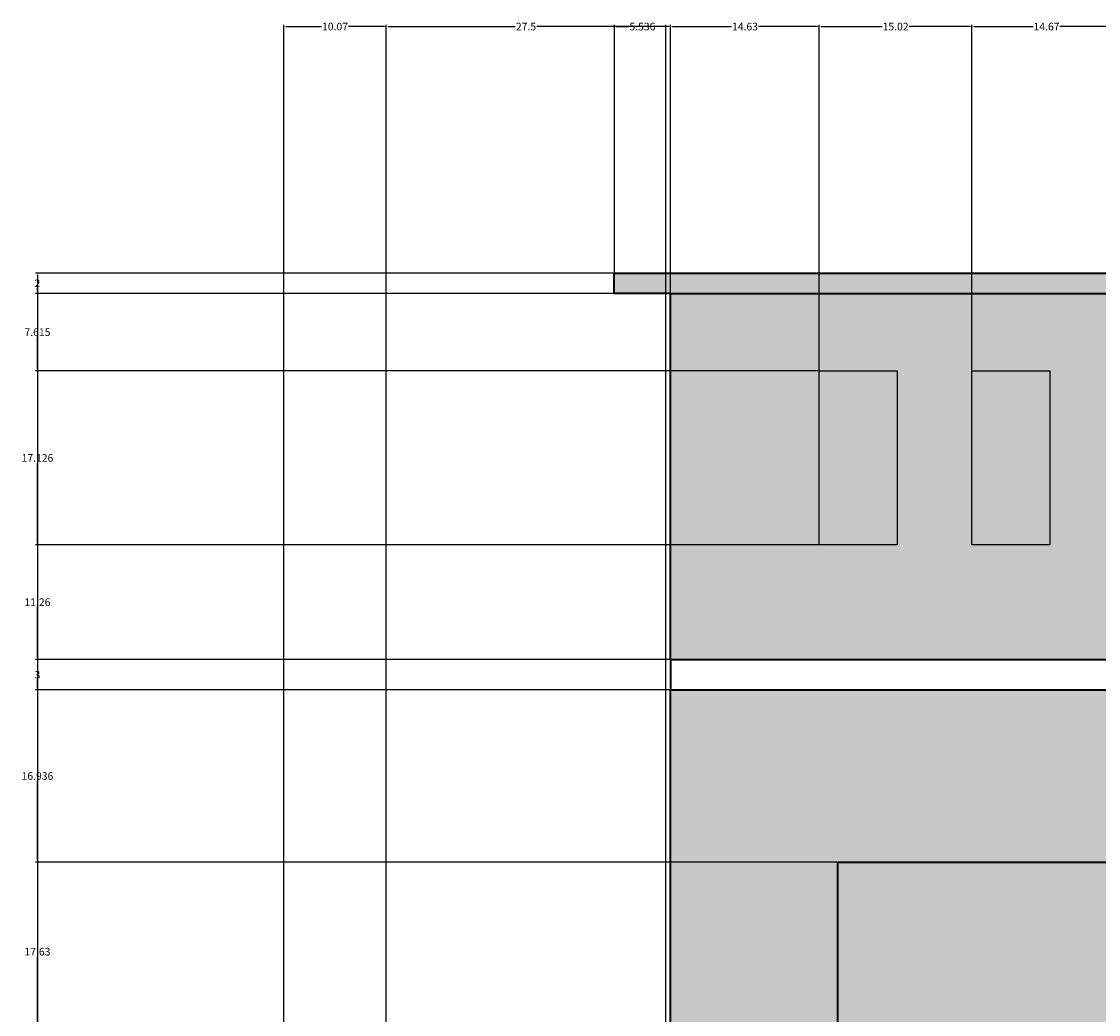
# Model space of a CAD drawing. Units: inches. Extents: x 62 to 566, y 66 to 528.
# Tile 9 of 20: x 62 to 168, y 430 to 528. Entities that reach past the tile are written whole.
import ezdxf

# ---------------------------------------------------------------- set-up
doc = ezdxf.new("R2010")
doc.units = ezdxf.units.IN
doc.header["$MEASUREMENT"] = 0
for name, color, linetype, lineweight in [('A-ANNO-DIMS', 2, 'Continuous', 18), ('A-ELEV', 7, 'Continuous', 35), ('A-GLAZ', 3, 'Continuous', 25), ('A-WALL-PATT', 8, 'Continuous', 13)]:
    doc.layers.add(name, color=color, linetype=linetype, lineweight=lineweight)
doc.styles.get("Standard").update_dxf_attribs({"font": 'arial.ttf'})
doc.dimstyles.get("Standard").update_dxf_attribs({"dimtxt": 0.75, "dimasz": 0.18, "dimexe": 0.18, "dimexo": 0.0625, "dimgap": 0.09, "dimtad": 0, "dimtih": 1, "dimtoh": 1, "dimdec": 4, "dimzin": 0, "dimdsep": 46, "dimlunit": 4, "dimtxsty": 'Standard', "dimcen": 0.09, "dimadec": 0, "dimazin": 0, "dimtfac": 1, "dimtdec": 4, "dimtofl": 0, "dimtmove": 0, "dimatfit": 3, "dimfxl": 1, "dimtolj": 1, "dimtzin": 0, "dimarcsym": 0})

# ---------------------------------------------------------------- blocks, each defined once
blk = doc.blocks.new('VENT-OPENING')
blk.add_lwpolyline([(0, 17.13), (7.66, 17.13), (7.66, 0), (0, 0)], close=True)
blk = doc.blocks.new('*D14')
at = {"layer": 'A-ANNO-DIMS', "color": 0, "lineweight": -2, "transparency": 16777216}
for p, q in [((87.9, 174.13), (87.9, 527.47)), ((88.08, 527.29), (91.61, 527.29)), ((97.79, 527.29), (94.25, 527.29)), ((97.97, 174.13), (97.97, 527.47))]:
    blk.add_line(p, q, dxfattribs=at)
at = {"layer": 'A-ANNO-DIMS', "color": 0, "transparency": 16777216}
for points in [[(88.08, 527.32), (88.08, 527.26), (87.9, 527.29)], [(97.79, 527.32), (97.79, 527.26), (97.97, 527.29)]]:
    blk.add_solid(points, dxfattribs=at)
at = {"layer": 'Defpoints', "color": 0, "transparency": 16777216}
for p in [(97.97, 527.29), (87.9, 174.07), (97.97, 174.07)]:
    blk.add_point(p, dxfattribs=at)
at = {"layer": 'A-ANNO-DIMS', "color": 0, "transparency": 16777216, "insert": (92.93, 527.29), "char_height": 0.75, "attachment_point": 5}
blk.add_mtext('\\A1;10.07', dxfattribs=at)
blk = doc.blocks.new('*D15')
at = {"layer": 'A-ANNO-DIMS', "color": 0, "lineweight": -2, "transparency": 16777216}
for p, q in [((97.97, 174.13), (97.97, 527.47)), ((98.15, 527.29), (110.64, 527.29)), ((125.28, 527.29), (112.79, 527.29)), ((125.46, 174.13), (125.46, 527.47))]:
    blk.add_line(p, q, dxfattribs=at)
at = {"layer": 'A-ANNO-DIMS', "color": 0, "transparency": 16777216}
for points in [[(98.15, 527.32), (98.15, 527.26), (97.97, 527.29)], [(125.28, 527.32), (125.28, 527.26), (125.46, 527.29)]]:
    blk.add_solid(points, dxfattribs=at)
at = {"layer": 'Defpoints', "color": 0, "transparency": 16777216}
for p in [(125.46, 527.29), (97.97, 174.07), (125.46, 174.07)]:
    blk.add_point(p, dxfattribs=at)
at = {"layer": 'A-ANNO-DIMS', "color": 0, "transparency": 16777216, "insert": (111.72, 527.29), "char_height": 0.75, "attachment_point": 5}
blk.add_mtext('\\A1;27.5', dxfattribs=at)
blk = doc.blocks.new('*D18')
at = {"layer": 'A-ANNO-DIMS', "color": 0, "lineweight": -2, "transparency": 16777216}
for p, q in [((120.34, 503.04), (63.47, 503.04)), ((63.65, 502.86), (63.65, 339.03)), ((63.65, 174.25), (63.65, 338.08)), ((87.83, 174.07), (63.47, 174.07))]:
    blk.add_line(p, q, dxfattribs=at)
at = {"layer": 'A-ANNO-DIMS', "color": 0, "transparency": 16777216}
for points in [[(63.62, 502.86), (63.68, 502.86), (63.65, 503.04)], [(63.62, 174.25), (63.68, 174.25), (63.65, 174.07)]]:
    blk.add_solid(points, dxfattribs=at)
at = {"layer": 'Defpoints', "color": 0, "transparency": 16777216}
for p in [(63.65, 503.04), (120.41, 503.04), (87.9, 174.07)]:
    blk.add_point(p, dxfattribs=at)
at = {"layer": 'A-ANNO-DIMS', "color": 0, "transparency": 16777216, "insert": (63.65, 338.55), "char_height": 0.75, "attachment_point": 5}
blk.add_mtext('\\A1;329', dxfattribs=at)
blk = doc.blocks.new('*D25')
at = {"layer": 'A-ANNO-DIMS', "color": 0, "lineweight": -2, "transparency": 16777216}
for p, q in [((120.41, 503.1), (120.41, 527.47)), ((120.59, 527.29), (121.82, 527.29)), ((125.76, 527.29), (124.53, 527.29)), ((125.94, 501.1), (125.94, 527.47))]:
    blk.add_line(p, q, dxfattribs=at)
at = {"layer": 'A-ANNO-DIMS', "color": 0, "transparency": 16777216}
for points in [[(120.59, 527.32), (120.59, 527.26), (120.41, 527.29)], [(125.76, 527.32), (125.76, 527.26), (125.94, 527.29)]]:
    blk.add_solid(points, dxfattribs=at)
at = {"layer": 'Defpoints', "color": 0, "transparency": 16777216}
for p in [(125.94, 527.29), (120.41, 503.04), (125.94, 501.04)]:
    blk.add_point(p, dxfattribs=at)
at = {"layer": 'A-ANNO-DIMS', "color": 0, "transparency": 16777216, "insert": (123.17, 527.29), "char_height": 0.75, "attachment_point": 5}
blk.add_mtext('\\A1;5.536', dxfattribs=at)
blk = doc.blocks.new('*D26')
at = {"layer": 'A-ANNO-DIMS', "color": 0, "lineweight": -2, "transparency": 16777216}
for p, q in [((125.94, 501.1), (125.94, 527.47)), ((126.12, 527.29), (131.94, 527.29)), ((140.39, 527.29), (134.58, 527.29)), ((140.57, 493.49), (140.57, 527.47))]:
    blk.add_line(p, q, dxfattribs=at)
at = {"layer": 'A-ANNO-DIMS', "color": 0, "transparency": 16777216}
for points in [[(126.12, 527.32), (126.12, 527.26), (125.94, 527.29)], [(140.39, 527.32), (140.39, 527.26), (140.57, 527.29)]]:
    blk.add_solid(points, dxfattribs=at)
at = {"layer": 'Defpoints', "color": 0, "transparency": 16777216}
for p in [(140.57, 527.29), (125.94, 501.04), (140.57, 493.43)]:
    blk.add_point(p, dxfattribs=at)
at = {"layer": 'A-ANNO-DIMS', "color": 0, "transparency": 16777216, "insert": (133.26, 527.29), "char_height": 0.75, "attachment_point": 5}
blk.add_mtext('\\A1;14.63', dxfattribs=at)
blk = doc.blocks.new('*D27')
at = {"layer": 'A-ANNO-DIMS', "color": 0, "lineweight": -2, "transparency": 16777216}
for p, q in [((140.57, 493.49), (140.57, 527.47)), ((140.75, 527.29), (146.76, 527.29)), ((155.41, 527.29), (149.4, 527.29)), ((155.59, 493.49), (155.59, 527.47))]:
    blk.add_line(p, q, dxfattribs=at)
at = {"layer": 'A-ANNO-DIMS', "color": 0, "transparency": 16777216}
for points in [[(140.75, 527.32), (140.75, 527.26), (140.57, 527.29)], [(155.41, 527.32), (155.41, 527.26), (155.59, 527.29)]]:
    blk.add_solid(points, dxfattribs=at)
at = {"layer": 'Defpoints', "color": 0, "transparency": 16777216}
for p in [(155.59, 527.29), (140.57, 493.43), (155.59, 493.43)]:
    blk.add_point(p, dxfattribs=at)
at = {"layer": 'A-ANNO-DIMS', "color": 0, "transparency": 16777216, "insert": (148.08, 527.29), "char_height": 0.75, "attachment_point": 5}
blk.add_mtext('\\A1;15.02', dxfattribs=at)
blk = doc.blocks.new('*D28')
at = {"layer": 'A-ANNO-DIMS', "color": 0, "lineweight": -2, "transparency": 16777216}
for p, q in [((155.59, 493.49), (155.59, 527.47)), ((155.77, 527.29), (161.61, 527.29)), ((170.08, 527.29), (164.25, 527.29)), ((170.26, 493.84), (170.26, 527.47))]:
    blk.add_line(p, q, dxfattribs=at)
at = {"layer": 'A-ANNO-DIMS', "color": 0, "transparency": 16777216}
for points in [[(155.77, 527.32), (155.77, 527.26), (155.59, 527.29)], [(170.08, 527.32), (170.08, 527.26), (170.26, 527.29)]]:
    blk.add_solid(points, dxfattribs=at)
at = {"layer": 'Defpoints', "color": 0, "transparency": 16777216}
for p in [(170.26, 527.29), (170.26, 493.78), (155.59, 493.43)]:
    blk.add_point(p, dxfattribs=at)
at = {"layer": 'A-ANNO-DIMS', "color": 0, "transparency": 16777216, "insert": (162.93, 527.29), "char_height": 0.75, "attachment_point": 5}
blk.add_mtext('\\A1;14.67', dxfattribs=at)
blk = doc.blocks.new('*D35')
at = {"layer": 'A-ANNO-DIMS', "color": 0, "lineweight": -2, "transparency": 16777216}
for p, q in [((125.94, 461.98), (125.94, 65.94)), ((142.39, 445.04), (142.39, 65.94)), ((126.12, 66.12), (132.55, 66.12)), ((142.21, 66.12), (135.77, 66.12))]:
    blk.add_line(p, q, dxfattribs=at)
at = {"layer": 'A-ANNO-DIMS', "color": 0, "transparency": 16777216}
for points in [[(126.12, 66.15), (126.12, 66.09), (125.94, 66.12)], [(142.21, 66.15), (142.21, 66.09), (142.39, 66.12)]]:
    blk.add_solid(points, dxfattribs=at)
at = {"layer": 'Defpoints', "color": 0, "transparency": 16777216}
for p in [(125.94, 462.04), (142.39, 445.11), (142.39, 66.12)]:
    blk.add_point(p, dxfattribs=at)
at = {"layer": 'A-ANNO-DIMS', "color": 0, "transparency": 16777216, "insert": (134.16, 66.12), "char_height": 0.75, "attachment_point": 5}
blk.add_mtext('\\A1;16.443', dxfattribs=at)
blk = doc.blocks.new('*D36')
at = {"layer": 'A-ANNO-DIMS', "color": 0, "lineweight": -2, "transparency": 16777216}
for p, q in [((142.39, 445.04), (142.39, 65.94)), ((163.65, 427.41), (163.65, 65.94)), ((142.57, 66.12), (151.66, 66.12)), ((163.47, 66.12), (154.38, 66.12))]:
    blk.add_line(p, q, dxfattribs=at)
at = {"layer": 'A-ANNO-DIMS', "color": 0, "transparency": 16777216}
for points in [[(142.57, 66.15), (142.57, 66.09), (142.39, 66.12)], [(163.47, 66.15), (163.47, 66.09), (163.65, 66.12)]]:
    blk.add_solid(points, dxfattribs=at)
at = {"layer": 'Defpoints', "color": 0, "transparency": 16777216}
for p in [(142.39, 445.11), (163.65, 427.48), (163.65, 66.12)]:
    blk.add_point(p, dxfattribs=at)
at = {"layer": 'A-ANNO-DIMS', "color": 0, "transparency": 16777216, "insert": (153.02, 66.12), "char_height": 0.75, "attachment_point": 5}
blk.add_mtext('\\A1;21.27', dxfattribs=at)
blk = doc.blocks.new('*D45')
at = {"layer": 'A-ANNO-DIMS', "color": 0, "lineweight": -2, "transparency": 16777216}
for p, q in [((142.32, 445.11), (63.47, 445.11)), ((63.65, 444.93), (63.65, 436.76)), ((63.65, 427.66), (63.65, 435.82)), ((163.59, 427.48), (63.47, 427.48))]:
    blk.add_line(p, q, dxfattribs=at)
at = {"layer": 'A-ANNO-DIMS', "color": 0, "transparency": 16777216}
for points in [[(63.62, 444.93), (63.68, 444.93), (63.65, 445.11)], [(63.62, 427.66), (63.68, 427.66), (63.65, 427.48)]]:
    blk.add_solid(points, dxfattribs=at)
at = {"layer": 'Defpoints', "color": 0, "transparency": 16777216}
for p in [(63.65, 445.11), (142.39, 445.11), (163.65, 427.48)]:
    blk.add_point(p, dxfattribs=at)
at = {"layer": 'A-ANNO-DIMS', "color": 0, "transparency": 16777216, "insert": (63.65, 436.29), "char_height": 0.75, "attachment_point": 5}
blk.add_mtext('\\A1;17.63', dxfattribs=at)
blk = doc.blocks.new('*D46')
at = {"layer": 'A-ANNO-DIMS', "color": 0, "lineweight": -2, "transparency": 16777216}
for p, q in [((125.88, 462.04), (63.47, 462.04)), ((63.65, 461.86), (63.65, 454.05)), ((63.65, 445.29), (63.65, 453.1)), ((142.32, 445.11), (63.47, 445.11))]:
    blk.add_line(p, q, dxfattribs=at)
at = {"layer": 'A-ANNO-DIMS', "color": 0, "transparency": 16777216}
for points in [[(63.62, 461.86), (63.68, 461.86), (63.65, 462.04)], [(63.62, 445.29), (63.68, 445.29), (63.65, 445.11)]]:
    blk.add_solid(points, dxfattribs=at)
at = {"layer": 'Defpoints', "color": 0, "transparency": 16777216}
for p in [(63.65, 462.04), (125.94, 462.04), (142.39, 445.11)]:
    blk.add_point(p, dxfattribs=at)
at = {"layer": 'A-ANNO-DIMS', "color": 0, "transparency": 16777216, "insert": (63.65, 453.57), "char_height": 0.75, "attachment_point": 5}
blk.add_mtext('\\A1;16.936', dxfattribs=at)
blk = doc.blocks.new('*D47')
at = {"layer": 'A-ANNO-DIMS', "color": 0, "lineweight": -2, "transparency": 16777216}
for p, q in [((125.88, 465.04), (63.47, 465.04)), ((63.65, 464.86), (63.65, 464.02)), ((63.65, 462.22), (63.65, 463.07)), ((125.88, 462.04), (63.47, 462.04))]:
    blk.add_line(p, q, dxfattribs=at)
at = {"layer": 'A-ANNO-DIMS', "color": 0, "transparency": 16777216}
for points in [[(63.62, 464.86), (63.68, 464.86), (63.65, 465.04)], [(63.62, 462.22), (63.68, 462.22), (63.65, 462.04)]]:
    blk.add_solid(points, dxfattribs=at)
at = {"layer": 'Defpoints', "color": 0, "transparency": 16777216}
for p in [(63.65, 465.04), (125.94, 465.04), (125.94, 462.04)]:
    blk.add_point(p, dxfattribs=at)
at = {"layer": 'A-ANNO-DIMS', "color": 0, "transparency": 16777216, "insert": (63.65, 463.54), "char_height": 0.75, "attachment_point": 5}
blk.add_mtext('\\A1;3', dxfattribs=at)
blk = doc.blocks.new('*D48')
at = {"layer": 'A-ANNO-DIMS', "color": 0, "lineweight": -2, "transparency": 16777216}
for p, q in [((140.51, 476.3), (63.47, 476.3)), ((63.65, 476.12), (63.65, 471.14)), ((63.65, 465.22), (63.65, 470.2)), ((125.88, 465.04), (63.47, 465.04))]:
    blk.add_line(p, q, dxfattribs=at)
at = {"layer": 'A-ANNO-DIMS', "color": 0, "transparency": 16777216}
for points in [[(63.62, 476.12), (63.68, 476.12), (63.65, 476.3)], [(63.62, 465.22), (63.68, 465.22), (63.65, 465.04)]]:
    blk.add_solid(points, dxfattribs=at)
at = {"layer": 'Defpoints', "color": 0, "transparency": 16777216}
for p in [(63.65, 476.3), (140.57, 476.3), (125.94, 465.04)]:
    blk.add_point(p, dxfattribs=at)
at = {"layer": 'A-ANNO-DIMS', "color": 0, "transparency": 16777216, "insert": (63.65, 470.67), "char_height": 0.75, "attachment_point": 5}
blk.add_mtext('\\A1;11.26', dxfattribs=at)
blk = doc.blocks.new('*D49')
at = {"layer": 'A-ANNO-DIMS', "color": 0, "lineweight": -2, "transparency": 16777216}
for p, q in [((140.51, 493.43), (63.47, 493.43)), ((63.65, 493.25), (63.65, 485.34)), ((63.65, 476.48), (63.65, 484.39)), ((140.51, 476.3), (63.47, 476.3))]:
    blk.add_line(p, q, dxfattribs=at)
at = {"layer": 'A-ANNO-DIMS', "color": 0, "transparency": 16777216}
for points in [[(63.62, 493.25), (63.68, 493.25), (63.65, 493.43)], [(63.62, 476.48), (63.68, 476.48), (63.65, 476.3)]]:
    blk.add_solid(points, dxfattribs=at)
at = {"layer": 'Defpoints', "color": 0, "transparency": 16777216}
for p in [(63.65, 493.43), (140.57, 493.43), (140.57, 476.3)]:
    blk.add_point(p, dxfattribs=at)
at = {"layer": 'A-ANNO-DIMS', "color": 0, "transparency": 16777216, "insert": (63.65, 484.86), "char_height": 0.75, "attachment_point": 5}
blk.add_mtext('\\A1;17.126', dxfattribs=at)
blk = doc.blocks.new('*D50')
at = {"layer": 'A-ANNO-DIMS', "color": 0, "lineweight": -2, "transparency": 16777216}
for p, q in [((125.88, 501.04), (63.47, 501.04)), ((63.65, 500.86), (63.65, 497.71)), ((63.65, 493.61), (63.65, 496.76)), ((140.51, 493.43), (63.47, 493.43))]:
    blk.add_line(p, q, dxfattribs=at)
at = {"layer": 'A-ANNO-DIMS', "color": 0, "transparency": 16777216}
for points in [[(63.62, 500.86), (63.68, 500.86), (63.65, 501.04)], [(63.62, 493.61), (63.68, 493.61), (63.65, 493.43)]]:
    blk.add_solid(points, dxfattribs=at)
at = {"layer": 'Defpoints', "color": 0, "transparency": 16777216}
for p in [(63.65, 501.04), (125.94, 501.04), (140.57, 493.43)]:
    blk.add_point(p, dxfattribs=at)
at = {"layer": 'A-ANNO-DIMS', "color": 0, "transparency": 16777216, "insert": (63.65, 497.23), "char_height": 0.75, "attachment_point": 5}
blk.add_mtext('\\A1;7.615', dxfattribs=at)
blk = doc.blocks.new('*D51')
at = {"layer": 'A-ANNO-DIMS', "color": 0, "lineweight": -2, "transparency": 16777216}
for p, q in [((120.34, 503.04), (63.47, 503.04)), ((63.65, 502.86), (63.65, 502.51)), ((63.65, 501.22), (63.65, 501.58)), ((125.88, 501.04), (63.47, 501.04))]:
    blk.add_line(p, q, dxfattribs=at)
at = {"layer": 'A-ANNO-DIMS', "color": 0, "transparency": 16777216}
for points in [[(63.62, 502.86), (63.68, 502.86), (63.65, 503.04)], [(63.62, 501.22), (63.68, 501.22), (63.65, 501.04)]]:
    blk.add_solid(points, dxfattribs=at)
at = {"layer": 'Defpoints', "color": 0, "transparency": 16777216}
for p in [(63.65, 503.04), (120.41, 503.04), (125.94, 501.04)]:
    blk.add_point(p, dxfattribs=at)
at = {"layer": 'A-ANNO-DIMS', "color": 0, "transparency": 16777216, "insert": (63.65, 502.04), "char_height": 0.75, "attachment_point": 5}
blk.add_mtext('\\A1;2', dxfattribs=at)

msp = doc.modelspace()

# ---------------------------------------------------------------- hatches: boundary and pattern name
at = {"layer": 'A-WALL-PATT'}
h = msp.add_hatch(color=256, dxfattribs=at)
h.dxf.hatch_style = 1
h.paths.add_polyline_path([(416.0836, 462.0423), (125.9418, 462.0423), (125.9418, 414.3686), (125.9418, 270.3686), (125.9418, 126.3686), (142.3851, 126.3686), (142.3851, 270.3686), (142.3851, 414.3686), (142.3851, 445.1064), (284.2021, 445.1064), (416.0836, 445.1064)])
h.paths.add_polyline_path([(435.3945, 503.0423), (426.3652, 503.0423), (120.4058, 503.0423), (120.4058, 501.0423), (125.9418, 501.0423), (416.0836, 501.0423), (426.3652, 501.0423), (430.6938, 501.0423), (435.3945, 501.0423)])
h.paths.add_polyline_path([(439.6878, 352.4848), (392.4793, 352.4848), (392.4793, 307.4128), (217.2752, 307.4128), (217.2752, 295.4098), (217.2752, 271.4128), (272.0586, 271.4128), (439.6878, 271.4128)])
h.paths.add_polyline_path([(248.0143, 297.1682), (255.6783, 297.1682), (255.6783, 280.0423), (248.0143, 280.0423)], flags=16)
h.paths.add_polyline_path([(235.4641, 280.0423), (227.8001, 280.0423), (227.8001, 297.1682), (235.4641, 297.1682)], flags=16)
h.paths.add_polyline_path([(270.4427, 297.1682), (278.1067, 297.1682), (278.1067, 280.0423), (270.4427, 280.0423)], flags=16)
h.paths.add_polyline_path([(296.3755, 297.1682), (304.0395, 297.1682), (304.0395, 280.0423), (296.3755, 280.0423)], flags=16)
h.paths.add_polyline_path([(319.2543, 297.1682), (326.9183, 297.1682), (326.9183, 280.0423), (319.2543, 280.0423)], flags=16)
h.paths.add_polyline_path([(341.2622, 297.1682), (348.9262, 297.1682), (348.9262, 280.0423), (341.2622, 280.0423)], flags=16)
h.paths.add_polyline_path([(389.2857, 298.3985), (433.8102, 298.3985), (433.8102, 294.9497), (389.2857, 294.9497)], flags=16)
h.paths.add_polyline_path([(389.2857, 291.6038), (433.8102, 291.6038), (433.8102, 288.155), (389.2857, 288.155)], flags=16)
h.paths.add_polyline_path([(389.2857, 284.9607), (433.8102, 284.9607), (433.8102, 281.5119), (389.2857, 281.5119)], flags=16)
h.paths.add_polyline_path([(403.5849, 311.4736), (403.5849, 317.4388), (433.1636, 317.4388), (433.1636, 311.4736)], flags=16)
h.paths.add_polyline_path([(403.5849, 323.1329), (403.5849, 329.0982), (433.1636, 329.0982), (433.1636, 323.1329)], flags=16)
h.paths.add_polyline_path([(403.5849, 334.5211), (403.5849, 340.4863), (433.1636, 340.4863), (433.1636, 334.5211)], flags=16)
h.paths.add_polyline_path([(272.0586, 160.3545), (217.2752, 160.3545), (217.2752, 129.0504), (217.2752, 126.3686), (272.0586, 126.3686)], flags=17)
h.paths.add_polyline_path([(220.5897, 149.5749), (220.5897, 152.296), (267.7931, 152.296), (267.7931, 149.5749)], flags=16)
h.paths.add_polyline_path([(267.7931, 146.6724), (267.7931, 143.9513), (220.5897, 143.9513), (220.5897, 146.6724)], flags=16)
h.paths.add_polyline_path([(220.5897, 155.3799), (220.5897, 158.101), (267.7931, 158.101), (267.7931, 155.3799)], flags=16)
h.paths.add_polyline_path([(267.7931, 140.686), (267.7931, 137.9649), (220.5897, 137.9649), (220.5897, 140.686)], flags=16)
h.paths.add_polyline_path([(267.7931, 135.516), (267.7931, 132.7949), (220.5897, 132.7949), (220.5897, 135.516)], flags=16)
h = msp.add_hatch(dxfattribs=at)
h.set_pattern_fill('ANSI36', color=256, scale=8.8)
h.paths.add_polyline_path([(217.2752, 420.597), (169.0431, 420.597), (169.0431, 126.3686), (217.2752, 126.3686), (217.2752, 129.0504), (217.2752, 271.4128), (217.2752, 295.4128), (217.2752, 307.4128)])
h.paths.add_polyline_path([(282.3509, 501.0423), (125.9418, 501.0423), (125.9418, 465.0423), (282.3509, 465.0423)])
h.paths.add_polyline_path([(209.709, 476.6506), (202.045, 476.6506), (202.045, 493.7764), (209.709, 493.7764)], flags=16)
h.paths.add_polyline_path([(193.9913, 476.6506), (186.3273, 476.6506), (186.3273, 493.7764), (193.9913, 493.7764)], flags=16)
h.paths.add_polyline_path([(177.9243, 476.6506), (170.2603, 476.6506), (170.2603, 493.7764), (177.9243, 493.7764)], flags=16)
h.paths.add_polyline_path([(163.2545, 476.3015), (155.5905, 476.3015), (155.5905, 493.4274), (163.2545, 493.4274)], flags=16)
h.paths.add_polyline_path([(148.2354, 476.3015), (140.5713, 476.3015), (140.5713, 493.4274), (148.2354, 493.4274)], flags=16)
h.paths.add_polyline_path([(284.2021, 126.3686), (87.8962, 126.3686), (87.8962, 114.3686), (87.8962, 90.3686), (284.2021, 90.3686)])
h.paths.add_polyline_path([(474.1214, 126.3686), (396.433, 126.3686), (396.433, 90.3686), (474.1214, 90.3686)])
h = msp.add_hatch(color=256, dxfattribs=at)
h.dxf.hatch_style = 1
h.paths.add_polyline_path([(416.0836, 501.0423), (282.3509, 501.0423), (282.3509, 465.0423), (416.0836, 465.0423)])
h.paths.add_polyline_path([(284.2021, 420.597), (272.0586, 420.597), (272.0586, 309.5388), (272.0586, 307.4128), (284.2021, 307.4128)], flags=17)
h.paths.add_polyline_path([(284.2021, 445.1064), (142.3851, 445.1064), (142.3851, 414.3686), (142.3851, 270.3686), (142.3851, 126.3686), (163.6548, 126.3686), (163.6548, 270.5016), (163.6548, 414.5016), (163.6548, 427.4752), (284.2021, 427.4752)])
h.paths.add_polyline_path([(235.4641, 297.1682), (227.8001, 297.1682), (227.8001, 280.0423), (235.4641, 280.0423)], flags=17)
h.paths.add_polyline_path([(255.6783, 297.1682), (248.0143, 297.1682), (248.0143, 280.0423), (255.6783, 280.0423)], flags=17)
h.paths.add_polyline_path([(278.1067, 297.1682), (270.4427, 297.1682), (270.4427, 280.0423), (278.1067, 280.0423)], flags=17)
h.paths.add_polyline_path([(304.0395, 297.1682), (296.3755, 297.1682), (296.3755, 280.0423), (304.0395, 280.0423)])
h.paths.add_polyline_path([(326.9183, 297.1682), (319.2543, 297.1682), (319.2543, 280.0423), (326.9183, 280.0423)])
h.paths.add_polyline_path([(348.9262, 297.1682), (341.2622, 297.1682), (341.2622, 280.0423), (348.9262, 280.0423)])
h.paths.add_polyline_path([(433.8102, 284.9607), (389.2857, 284.9607), (389.2857, 281.5119), (433.8102, 281.5119)])
h.paths.add_polyline_path([(433.8102, 291.6038), (389.2857, 291.6038), (389.2857, 288.155), (433.8102, 288.155)])
h.paths.add_polyline_path([(433.8102, 298.3985), (389.2857, 298.3985), (389.2857, 294.9497), (433.8102, 294.9497)])
h.paths.add_polyline_path([(433.1636, 317.4388), (403.5849, 317.4388), (403.5849, 311.4736), (433.1636, 311.4736)])
h.paths.add_polyline_path([(433.1636, 329.0982), (403.5849, 329.0982), (403.5849, 323.1329), (433.1636, 323.1329)])
h.paths.add_polyline_path([(433.1636, 340.4863), (403.5849, 340.4863), (403.5849, 334.5211), (433.1636, 334.5211)])
h.paths.add_polyline_path([(284.2021, 271.4128), (272.0586, 271.4128), (272.0586, 160.3545), (272.0586, 126.3686), (284.2021, 126.3686)])
h.paths.add_polyline_path([(267.7931, 158.101), (220.5897, 158.101), (220.5897, 155.3799), (267.7931, 155.3799)], flags=17)
h.paths.add_polyline_path([(267.7931, 152.296), (220.5897, 152.296), (220.5897, 149.5749), (267.7931, 149.5749)], flags=17)
h.paths.add_polyline_path([(267.7931, 146.6724), (220.5897, 146.6724), (220.5897, 143.9513), (267.7931, 143.9513)], flags=17)
h.paths.add_polyline_path([(267.7931, 140.686), (220.5897, 140.686), (220.5897, 137.9649), (267.7931, 137.9649)], flags=17)
h.paths.add_polyline_path([(267.7931, 135.516), (220.5897, 135.516), (220.5897, 132.7949), (267.7931, 132.7949)], flags=17)
h.paths.add_polyline_path([(148.2354, 493.4274), (140.5713, 493.4274), (140.5713, 476.3015), (148.2354, 476.3015)])
h.paths.add_polyline_path([(163.2545, 493.4274), (155.5905, 493.4274), (155.5905, 476.3015), (163.2545, 476.3015)])
h.paths.add_polyline_path([(177.9243, 493.7764), (170.2603, 493.7764), (170.2603, 476.6506), (177.9243, 476.6506)])
h.paths.add_polyline_path([(193.9913, 493.7764), (186.3273, 493.7764), (186.3273, 476.6506), (193.9913, 476.6506)])
h.paths.add_polyline_path([(209.709, 493.7764), (202.045, 493.7764), (202.045, 476.6506), (209.709, 476.6506)])

# ---------------------------------------------------------------- linework, layer by layer
at = {"layer": 'A-ELEV'}
for p, q in [((120.4058, 501.0423), (120.4058, 503.0423)), ((120.4058, 503.0423), (426.3652, 503.0423)), ((125.9418, 501.0423), (120.4058, 501.0423)), ((125.9418, 465.0423), (125.9418, 501.0423)), ((125.9418, 501.0423), (416.0836, 501.0423)), ((125.9418, 465.0423), (416.0836, 465.0423)), ((125.9418, 465.0423), (125.9418, 462.0423)), ((125.9418, 414.3686), (125.9418, 462.0423)), ((125.9418, 462.0423), (416.0836, 462.0423)), ((142.3851, 414.3686), (142.3851, 445.1064)), ((142.3851, 445.1064), (284.2021, 445.1064))]:
    msp.add_line(p, q, dxfattribs=at)

# ---------------------------------------------------------------- block references
at = {"layer": 'A-GLAZ'}
for p in [(140.5713, 476.3015), (155.5905, 476.3015)]:
    msp.add_blockref('VENT-OPENING', p, dxfattribs=at)

# ---------------------------------------------------------------- dimensions: what is measured, and where the dimension line sits
at = {"layer": 'A-ANNO-DIMS'}
for base, p1, p2, override, picture, middle in [((97.967, 527.2923), (87.8962, 174.0659), (97.967, 174.0659), {"dimdec": 2, "dimlfac": 1, "dimrnd": 0, "dimzin": 0, "dimdsep": 46, "dimlunit": 2}, '*D14', (92.9316, 527.2923)), ((125.4645, 527.2923), (97.967, 174.0659), (125.4645, 174.0659), {"dimdec": 1, "dimlfac": 1, "dimrnd": 0, "dimzin": 0, "dimdsep": 46, "dimlunit": 2}, '*D15', (111.7157, 527.2923)), ((125.9418, 527.2923), (120.4058, 503.0423), (125.9418, 501.0423), {"dimdec": 3, "dimlfac": 1, "dimrnd": 0, "dimzin": 0, "dimdsep": 46, "dimlunit": 2}, '*D25', (123.1738, 527.2923)), ((140.5713, 527.2923), (125.9418, 501.0423), (140.5713, 493.4274), {"dimdec": 2, "dimlfac": 1, "dimrnd": 0, "dimzin": 0, "dimdsep": 46, "dimlunit": 2}, '*D26', (133.2566, 527.2923)), ((155.5905, 527.2923), (140.5713, 493.4274), (155.5905, 493.4274), {"dimdec": 2, "dimlfac": 1, "dimrnd": 0, "dimzin": 0, "dimdsep": 46, "dimlunit": 2}, '*D27', (148.0809, 527.2923)), ((170.2603, 527.2923), (155.5905, 493.4274), (170.2603, 493.7764), {"dimdec": 2, "dimlfac": 1, "dimrnd": 0, "dimzin": 0, "dimdsep": 46, "dimlunit": 2}, '*D28', (162.9254, 527.2923)), ((142.3851, 66.1186), (125.9418, 462.0423), (142.3851, 445.1064), {"dimdec": 3, "dimlfac": 1, "dimrnd": 0, "dimzin": 0, "dimdsep": 46, "dimlunit": 2}, '*D35', (134.1634, 66.1186)), ((163.6548, 66.1186), (142.3851, 445.1064), (163.6548, 427.4752), {"dimdec": 2, "dimlfac": 1, "dimrnd": 0, "dimzin": 0, "dimdsep": 46, "dimlunit": 2}, '*D36', (153.0199, 66.1186))]:
    dim = msp.add_linear_dim(base=base, p1=p1, p2=p2, dimstyle='Standard', override=override, dxfattribs=at)
    dim.commit()
    dim.dimension.update_dxf_attribs({"geometry": picture, "text_midpoint": middle})
for base, p1, p2, override, picture, middle in [((63.6462, 503.0423), (87.8962, 174.0659), (120.4058, 503.0423), {"dimdec": 0, "dimlfac": 1, "dimrnd": 0, "dimzin": 0, "dimdsep": 46, "dimlunit": 2}, '*D18', (63.6462, 338.5541)), ((63.6462, 503.0423), (125.9418, 501.0423), (120.4058, 503.0423), {"dimdec": 0, "dimlfac": 1, "dimrnd": 0, "dimzin": 0, "dimdsep": 46, "dimlunit": 2}, '*D51', (63.6462, 502.0423)), ((63.6462, 501.0423), (140.5713, 493.4274), (125.9418, 501.0423), {"dimdec": 3, "dimlfac": 1, "dimrnd": 0, "dimzin": 0, "dimdsep": 46, "dimlunit": 2}, '*D50', (63.6462, 497.2349)), ((63.6462, 493.4274), (140.5713, 476.3015), (140.5713, 493.4274), {"dimdec": 3, "dimlfac": 1, "dimrnd": 0, "dimzin": 0, "dimdsep": 46, "dimlunit": 2}, '*D49', (63.6462, 484.8645)), ((63.6462, 476.3015), (125.9418, 465.0423), (140.5713, 476.3015), {"dimdec": 2, "dimlfac": 1, "dimrnd": 0, "dimzin": 0, "dimdsep": 46, "dimlunit": 2}, '*D48', (63.6462, 470.6719)), ((63.6462, 465.0423), (125.9418, 462.0423), (125.9418, 465.0423), {"dimdec": 0, "dimlfac": 1, "dimrnd": 0, "dimzin": 0, "dimdsep": 46, "dimlunit": 2}, '*D47', (63.6462, 463.5423)), ((63.6462, 462.0423), (142.3851, 445.1064), (125.9418, 462.0423), {"dimdec": 3, "dimlfac": 1, "dimrnd": 0, "dimzin": 0, "dimdsep": 46, "dimlunit": 2}, '*D46', (63.6462, 453.5744)), ((63.6462, 445.1064), (163.6548, 427.4752), (142.3851, 445.1064), {"dimdec": 2, "dimlfac": 1, "dimrnd": 0, "dimzin": 0, "dimdsep": 46, "dimlunit": 2}, '*D45', (63.6462, 436.2908))]:
    dim = msp.add_linear_dim(base=base, p1=p1, p2=p2, angle=90, dimstyle='Standard', override=override, dxfattribs=at)
    dim.commit()
    dim.dimension.update_dxf_attribs({"geometry": picture, "text_midpoint": middle})

doc.saveas('drawing.dxf')
